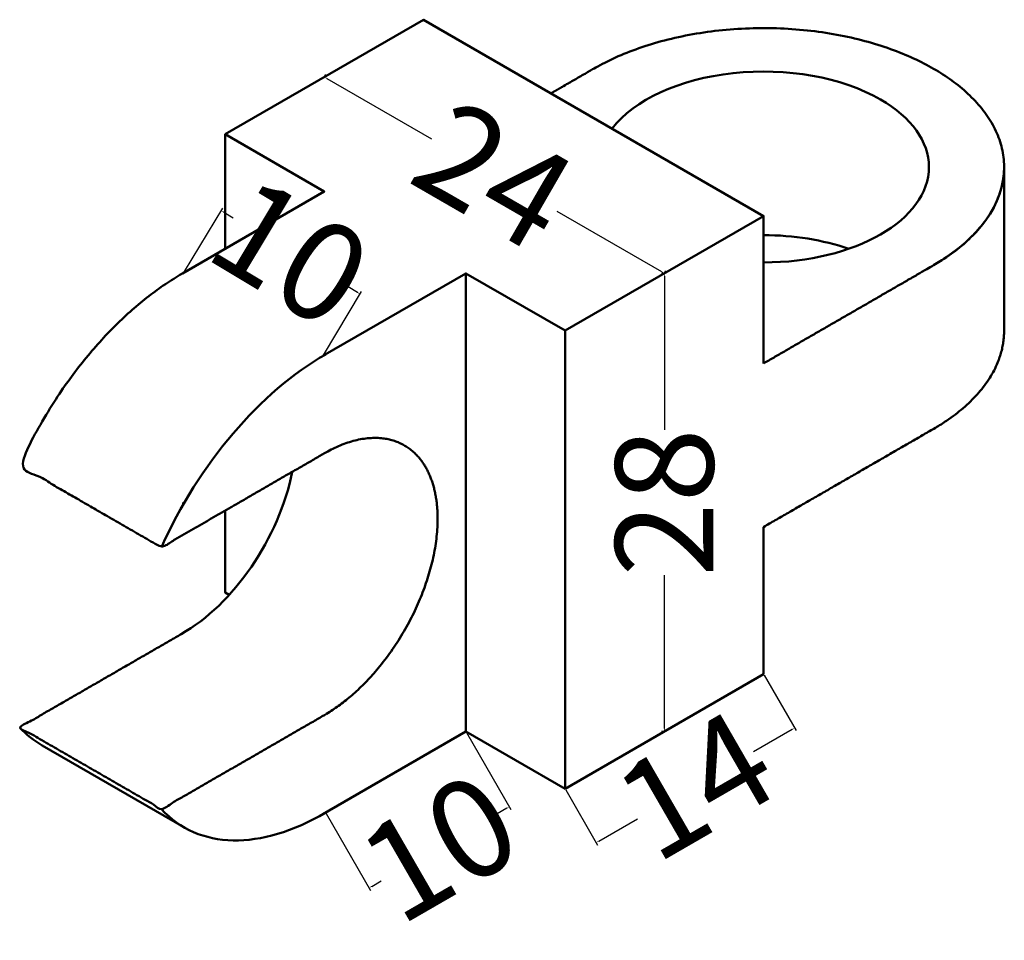
# Model space of a CAD drawing. Units: millimetres. Extents: x 28.4 to 88.6, y 53 to 109.3.
import ezdxf

# ---------------------------------------------------------------- set-up
doc = ezdxf.new("R2010")
doc.units = ezdxf.units.MM
doc.header["$MEASUREMENT"] = 0
doc.linetypes.add('CENTER', pattern=[2, 1.25, -0.25, 0.25, -0.25])
for name, color, linetype, lineweight in [('M-CNTR', 4, 'CENTER', 18), ('M-DIMS', 2, 'Continuous', 25), ('M-OUTL', 7, 'Continuous', 50)]:
    doc.layers.add(name, color=color, linetype=linetype, lineweight=lineweight)
doc.styles.get("Standard").update_dxf_attribs({"font": 'arial.ttf'})
doc.dimstyles.get("Standard").update_dxf_attribs({"dimtxt": 6, "dimasz": 0.18, "dimexe": 0.18, "dimexo": 0.0625, "dimgap": 0.09, "dimtad": 0, "dimtoh": 1, "dimdec": 0, "dimzin": 0, "dimdsep": 46, "dimtxsty": 'Standard', "dimcen": 0.09, "dimadec": 0, "dimazin": 0, "dimtfac": 1, "dimtdec": 0, "dimtofl": 0, "dimtmove": 0, "dimatfit": 3, "dimfxl": 1, "dimtolj": 1, "dimtzin": 0, "dimarcsym": 0})

# ---------------------------------------------------------------- blocks, each defined once
blk = doc.blocks.new('*D1')
at = {"layer": 'Defpoints', "color": 0, "transparency": 16777216}
for p in [(47.04, 105.798), (67.824, 93.798), (67.824, 93.798)]:
    blk.add_point(p, dxfattribs=at)
at = {"layer": 'M-DIMS', "color": 0, "lineweight": -2, "transparency": 16777216}
for p, q in [((47.071, 105.853), (47.13, 105.954)), ((47.196, 105.708), (53.599, 102.012)), ((67.669, 93.888), (61.265, 97.585)), ((67.856, 93.853), (67.914, 93.954))]:
    blk.add_line(p, q, dxfattribs=at)
at = {"layer": 'M-DIMS', "color": 0, "transparency": 16777216}
for points in [[(47.211, 105.734), (47.181, 105.682), (47.04, 105.798)], [(67.684, 93.914), (67.654, 93.862), (67.824, 93.798)]]:
    blk.add_solid(points, dxfattribs=at)
at = {"layer": 'M-DIMS', "color": 0, "transparency": 16777216, "insert": (57.432, 99.798), "char_height": 6, "attachment_point": 5, "rotation": 330}
blk.add_mtext('\\A1;24', dxfattribs=at)
blk = doc.blocks.new('*D2')
at = {"layer": 'Defpoints', "color": 0, "transparency": 16777216}
for p in [(67.824, 93.798), (67.824, 65.798), (67.824, 65.798)]:
    blk.add_point(p, dxfattribs=at)
at = {"layer": 'M-DIMS', "color": 0, "lineweight": -2, "transparency": 16777216}
for p, q in [((67.762, 93.798), (67.644, 93.798)), ((67.824, 93.618), (67.824, 84.243)), ((67.824, 65.978), (67.824, 75.354)), ((67.762, 65.798), (67.644, 65.798))]:
    blk.add_line(p, q, dxfattribs=at)
at = {"layer": 'M-DIMS', "color": 0, "transparency": 16777216}
for points in [[(67.794, 93.618), (67.854, 93.618), (67.824, 93.798)], [(67.794, 65.978), (67.854, 65.978), (67.824, 65.798)]]:
    blk.add_solid(points, dxfattribs=at)
at = {"layer": 'M-DIMS', "color": 0, "transparency": 16777216, "insert": (67.824, 79.798), "char_height": 6, "attachment_point": 5, "rotation": 90}
blk.add_mtext('\\A1;28', dxfattribs=at)
blk = doc.blocks.new('*D3')
at = {"layer": 'Defpoints', "color": 0, "transparency": 16777216}
for p in [(38.467, 93.848), (49.229, 92.534), (46.953, 88.748)]:
    blk.add_point(p, dxfattribs=at)
at = {"layer": 'M-DIMS', "color": 0, "lineweight": -2, "transparency": 16777216}
for p, q in [((38.499, 93.902), (40.835, 97.789)), ((40.897, 97.542), (41.476, 97.194)), ((46.985, 88.801), (49.321, 92.688)), ((49.074, 92.627), (48.495, 92.975))]:
    blk.add_line(p, q, dxfattribs=at)
at = {"layer": 'M-DIMS', "color": 0, "transparency": 16777216}
for points in [[(40.912, 97.568), (40.881, 97.516), (40.742, 97.635)], [(49.09, 92.652), (49.059, 92.601), (49.229, 92.534)]]:
    blk.add_solid(points, dxfattribs=at)
at = {"layer": 'M-DIMS', "color": 0, "transparency": 16777216, "insert": (44.985, 95.084), "char_height": 6, "attachment_point": 5, "rotation": 328.99257}
blk.add_mtext('\\A1;10', dxfattribs=at)
blk = doc.blocks.new('*D4')
at = {"layer": 'Defpoints', "color": 0, "transparency": 16777216}
for p in [(73.887, 69.298), (75.782, 66.016), (61.762, 62.298)]:
    blk.add_point(p, dxfattribs=at)
at = {"layer": 'M-DIMS', "color": 0, "lineweight": -2, "transparency": 16777216}
for p, q in [((73.918, 69.244), (75.872, 65.86)), ((75.626, 65.926), (73.264, 64.562)), ((61.794, 62.244), (63.747, 58.86)), ((63.813, 59.106), (66.175, 60.47))]:
    blk.add_line(p, q, dxfattribs=at)
at = {"layer": 'M-DIMS', "color": 0, "transparency": 16777216}
for points in [[(75.611, 65.952), (75.641, 65.9), (75.782, 66.016)], [(63.798, 59.132), (63.828, 59.08), (63.657, 59.016)]]:
    blk.add_solid(points, dxfattribs=at)
at = {"layer": 'M-DIMS', "color": 0, "transparency": 16777216, "insert": (69.72, 62.516), "char_height": 6, "attachment_point": 5, "rotation": 30}
blk.add_mtext('\\A1;14', dxfattribs=at)
blk = doc.blocks.new('*D5')
at = {"layer": 'Defpoints', "color": 0, "transparency": 16777216}
for p in [(55.7, 65.799), (47.127, 60.849), (58.355, 61.199)]:
    blk.add_point(p, dxfattribs=at)
at = {"layer": 'M-DIMS', "color": 0, "lineweight": -2, "transparency": 16777216}
for p, q in [((55.731, 65.744), (58.445, 61.043)), ((47.158, 60.795), (49.873, 56.093)), ((58.2, 61.109), (57.615, 60.771)), ((49.938, 56.339), (50.523, 56.677))]:
    blk.add_line(p, q, dxfattribs=at)
at = {"layer": 'M-DIMS', "color": 0, "transparency": 16777216}
for points in [[(58.185, 61.135), (58.215, 61.083), (58.355, 61.199)], [(49.923, 56.365), (49.953, 56.313), (49.783, 56.249)]]:
    blk.add_solid(points, dxfattribs=at)
at = {"layer": 'M-DIMS', "color": 0, "transparency": 16777216, "insert": (54.069, 58.724), "char_height": 6, "attachment_point": 5, "rotation": 30}
blk.add_mtext('\\A1;10', dxfattribs=at)

msp = doc.modelspace()

# ---------------------------------------------------------------- linework, layer by layer
at = {"layer": 'M-CNTR'}
msp.add_line((38.38, 79.798), (38.38, 79.596), dxfattribs=at)
at = {"layer": 'M-OUTL'}
for p, q in [((40.978, 95.298), (40.978, 102.298)), ((73.887, 88.298), (73.887, 97.298)), ((46.953, 88.748), (55.7, 93.798)), ((61.762, 90.298), (61.762, 62.298)), ((73.887, 69.298), (73.887, 78.298)), ((61.762, 62.298), (73.887, 69.298)), ((61.762, 62.298), (55.7, 65.798)), ((38.467, 59.949), (29.806, 64.949))]:
    msp.add_line(p, q, dxfattribs=at)
for points in [[(38.38, 93.798), (47.04, 98.798), (40.978, 102.298), (53.102, 109.298), (73.887, 97.298), (61.762, 90.298), (55.7, 93.798), (55.7, 65.799), (46.953, 60.749)], [(41.23, 74.153), (40.978, 74.298), (40.978, 79.298)]]:
    msp.add_lwpolyline(points, dxfattribs=at)
for centre, major_axis, start_param, end_param in [((73.887, 100.298), (10.104, 0), 0.785398, 2.728363), ((73.887, 100.298), (10.104, 0), 0, 0.785398), ((73.887, 100.298), (10.104, 0), 4.712389, 6.283185), ((73.887, 100.298), (14.697, 0), 5.497787, 6.283185), ((73.887, 90.298), (10.104, 0), 1.029612, 1.570796), ((47.04, 74.798), (-8.573, -14.849), 3.919812, 4.889597), ((38.38, 79.798), (-4.899, -8.485), 0.772835, 2.103433), ((38.38, 79.798), (-4.899, -8.485), 7.068474, 7.068583), ((38.38, 79.798), (8.573, 14.849), 2.96444, 3.141593), ((47.04, 74.798), (-8.573, -14.849), 6.105978, 7.075762)]:
    msp.add_ellipse(centre, major_axis=major_axis, ratio=0.57735, start_param=start_param, end_param=end_param, dxfattribs=at)
for points, weights, knots in [([(73.887, 88.298), (79.083, 91.298), (84.279, 94.298), (94.671, 100.298), (84.279, 106.298), (73.887, 112.298), (63.494, 106.298), (62.195, 105.548), (60.896, 104.798)], [1, 1, 1, 0.707106781187, 1, 0.707106781187, 1, 1, 1], [0, 0, 0, 1, 1, 2.570796, 2.570796, 4.141593, 4.141593, 5.141593, 5.141593, 5.141593]), ([(73.887, 78.298), (79.083, 81.298), (84.279, 84.298), (88.584, 86.784), (88.584, 90.298), (88.584, 95.298), (88.584, 100.298)], [1, 1, 1, 0.923879532511, 1, 1, 1], [0, 0, 0, 1, 1, 1.785398, 1.785398, 2.785398, 2.785398, 2.785398]), ([(38.467, 93.848), (32.079, 90.213), (28.429, 82.053), (32.759, 79.553), (37.09, 77.053), (42.021, 79.9), (46.953, 82.748), (50.991, 85.138), (53.025, 82.283), (55.059, 79.428), (53.025, 74.225), (50.991, 69.022), (46.953, 66.749), (42.021, 63.902), (37.09, 61.054), (32.759, 63.554), (28.429, 66.054), (33.404, 68.926), (38.38, 71.798)], [1, 0.884725132729, 1, 1, 1, 1, 1, 0.863923905235, 1, 0.863923905235, 1, 0.863923905235, 1, 1, 1, 1, 1, 1, 1], [0, 0, 0, 0.969785, 0.969785, 1.969785, 1.969785, 2.969785, 2.969785, 4.025358, 4.025358, 5.080931, 5.080931, 6.136504, 6.136504, 7.136504, 7.136504, 8.136504, 8.136504, 9.136504, 9.136504, 9.136504])]:
    msp.add_rational_spline(points, weights, degree=2, knots=knots, dxfattribs=at)

# ---------------------------------------------------------------- dimensions: what is measured, and where the dimension line sits
at = {"layer": 'M-DIMS'}
for p1, p2, distance, picture, middle in [((47.04, 105.798), (67.824, 93.798), 0, '*D1', (57.432, 99.798)), ((38.467, 93.848), (46.953, 88.748), 4.418, '*D3', (44.985, 95.084)), ((67.824, 93.798), (67.824, 65.798), 0, '*D2', (67.824, 79.798)), ((61.762, 62.298), (73.887, 69.298), -3.79, '*D4', (69.72, 62.516)), ((47.127, 60.849), (55.7, 65.799), -5.311, '*D5', (54.069, 58.724))]:
    dim = msp.add_aligned_dim(p1=p1, p2=p2, distance=distance, dimstyle='Standard', override={"dimclrd": 0, "dimclre": 0, "dimclrt": 0}, dxfattribs=at)
    dim.commit()
    dim.dimension.update_dxf_attribs({"geometry": picture, "text_midpoint": middle})

doc.saveas('drawing.dxf')
